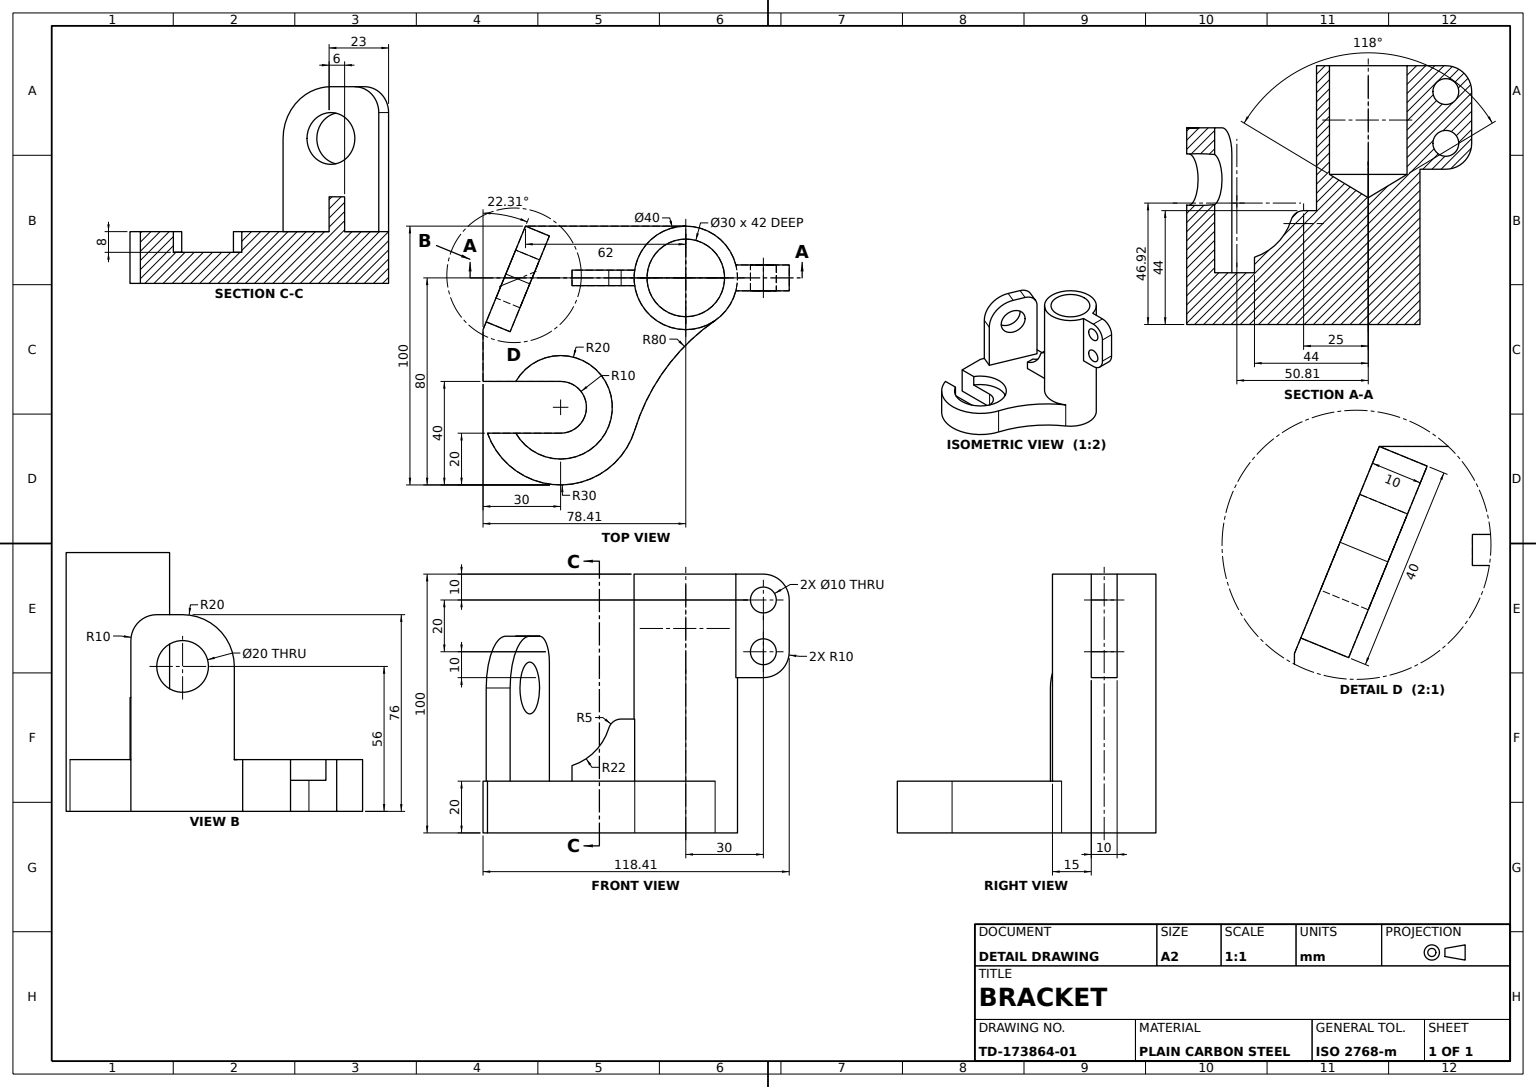
SolidWorks part; units mm, degrees
material "Plain Carbon Steel"
ref_plane "Front Plane" through (0, 0, 0) normal (0, 0, 1) x (1, 0, 0)
ref_plane "Top Plane" through (0, 0, 0) normal (0, 1, 0) x (1, 0, 0)
ref_plane "Right Plane" through (0, 0, 0) normal (1, 0, 0) x (0, 0, -1)
sketch "Column Profile Sketch" plane through (0, 0, 0) normal (0, 1, 0) x (1, 0, 0)
  circle A0 centre (0, 0) radius 20
  dimension "D1" = 20
extrude "Column Boss" add sketch "Column Profile Sketch" along normal blind 100
sketch "Base Arm Profile Sketch" plane through (0, 0, 0) normal (0, 1, 0) x (1, 0, 0)
  line L0 (0, 20) -> (-62, 20)
  line L1 (-62, 20) -> (-78.41, -20)
  line L2 (-78.41, -20) -> (-78.41, -50)
  circle A0 centre (0, 0) radius 20 construction
  arc A1 (-78.41, -50) -> (-19.7371, -58.8242) centre (-48.41, -50) ccw
  arc A2 (-19.7371, -58.8242) -> (11.3448, -16.4711) centre (56.7239, -82.3553) cw
  arc A3 (0, 20) -> (11.3448, -16.4711) centre (0, 0) ccw
  dimension "D1" = 30
  dimension "D6" = 80
  dimension "D2" = 40
  dimension "D3" = 78.41
  dimension "D4" = 62
  dimension "D5" = 50
extrude "Base Arm Plate" add sketch "Base Arm Profile Sketch" along normal blind 20
hole_wizard "Column Bore Ø30" positions "3DSketch1" profile "Sketch6" hole size "Ø25.5" standard "ANSI Metric"
sketch3d "3DSketch1"
  circle A0 centre (0, 100, 0) radius 20 construction
  point P0 (0, 100, 0)
  point P5 (0, 120, 0)
sketch "Sketch6" plane through (0, 100, 0) normal (1, 0, 0) x (0, 0, 1)
  line L0 (0, 0) -> (0, 51.0129)
  line L1 (0, 51.0129) -> (15, 42)
  line L2 (15, 42) -> (15, 0)
  line L5 (15, 0) -> (0, 0)
  line L10 (0, 51.0129) -> (-15, 42) construction
  line L11 (0, -6.35) -> (0, 107.95) construction
  dimension "Hole Dia." = 30
  dimension "Hole Depth" = 42
  dimension "Drill Angle" = 118
sketch "Hook Guide Block Sketch" plane through (-60.0913, 0, -24.6525) normal (-0.9252, 0, -0.3796) x (-0.3796, 0, 0.9252)
  line L0 (5.0288, 20) -> (5.0288, 66)
  line L1 (15.0288, 76) -> (25.0288, 76)
  line L2 (45.0288, 56) -> (45.0288, 20)
  line L3 (5.0288, 20) -> (48.264, 20) construction
  line L4 (45.0288, 20) -> (5.0288, 20)
  arc A0 (5.0288, 66) -> (15.0288, 76) centre (15.0288, 66) cw
  arc A1 (25.0288, 76) -> (45.0288, 56) centre (25.0288, 56) cw
  circle A2 centre (25.0288, 56) radius 10
  dimension "D2" = 10
  dimension "D3" = 20
  dimension "D4" = 20
  dimension "D1" = 56
  dimension "D5" = 40
extrude "Hook Guide Block" add sketch "Hook Guide Block Sketch" against normal blind 10
sketch "Hook Slot Sketch" plane through (0, 20, 0) normal (0, 1, 0) x (1, 0, 0)
  line L0 (-48.41, -40) -> (-78.41, -40)
  line L1 (-48.41, -60) -> (-78.41, -60)
  line L2 (-78.41, -60) -> (-78.41, -40)
  line L3 (-78.41, -20) -> (-78.41, -50) construction
  arc A0 (-48.41, -60) -> (-48.41, -40) centre (-48.41, -50) ccw
  arc A1 (-78.41, -50) -> (-19.7371, -58.8242) centre (-48.41, -50) ccw construction
  dimension "D1" = 20
extrude "Hook Slot Cut" cut sketch "Hook Slot Sketch" against normal through all
sketch "Hook Recess Sketch" plane through (0, 20, 0) normal (0, 1, 0) x (1, 0, 0)
  circle A0 centre (-48.41, -50) radius 20
  arc A1 (-76.6943, -60) -> (-19.7371, -58.8242) centre (-48.41, -50) ccw construction
  dimension "D1" = 20
extrude "Hook Recess Ø20" cut sketch "Hook Recess Sketch" against normal blind 8
sketch "Clamp Lug Sketch" plane through (0, 100, 0) normal (0, 1, 0) x (1, 0, 0)
  line L1 (18.522, 5) -> (40, 5)
  line L2 (18.522, 5) -> (18.522, -5)
  line L3 (18.522, -5) -> (40, -5)
  line L4 (40, 5) -> (40, -5)
  circle A0 centre (0, 0) radius 15 construction
  point P4 (18.522, 0)
  dimension "D1" = 10
  dimension "D2" = 40
  dimension "D3" = 18.522
extrude "Clamp Lug" add sketch "Clamp Lug Sketch" against normal blind 40
fillet "Clamp Lug Fillet R10" radius 10 2 edges at (40, 60, 0) (40, 100, 0)
sketch "Clamp Holes Sketch" plane through (0, 0, 5) normal (0, 0, 1) x (1, 0, 0)
  circle A0 centre (30, 90) radius 5
  circle A1 centre (30, 70) radius 5
  arc A2 (40, 90) -> (30, 100) centre (30, 90) ccw construction
  arc A3 (30, 60) -> (40, 70) centre (30, 70) ccw construction
  dimension "D1" = 10
extrude "Clamp Holes 2xØ10" cut sketch "Clamp Holes Sketch" against normal blind 40
sketch "Eye Lug Sketch" plane through (0, 0, 0) normal (0, 0, 1) x (1, 0, 0)
  line L0 (-44, 20) -> (-44, 26)
  line L1 (-19.7371, 20) -> (-76.6943, 20) construction
  line L2 (-20, 44) -> (-25, 44)
  line L3 (-20, 100) -> (-20, 20) construction
  line L5 (15, 100) -> (-15, 100) construction
  line L6 (-44, 20) -> (-17, 20)
  line L7 (11.3448, 20) -> (-19.7371, 20) construction
  line L8 (-17, 20) -> (-17, 44)
  line L9 (-17, 44) -> (-20, 44)
  arc A0 (-44, 26) -> (-29.7801, 40.4664) centre (-50.8127, 46.9186) ccw
  arc A1 (-25, 44) -> (-29.7801, 40.4664) centre (-25, 39) ccw
  dimension "D3" = 5
  dimension "D1" = 22
  dimension "D2" = 44
  dimension "D4" = 6
  dimension "D5" = 61
  dimension "D6" = 25
  dimension "D7" = 3
extrude "Eye Lug" add sketch "Eye Lug Sketch" along normal mid plane 6
